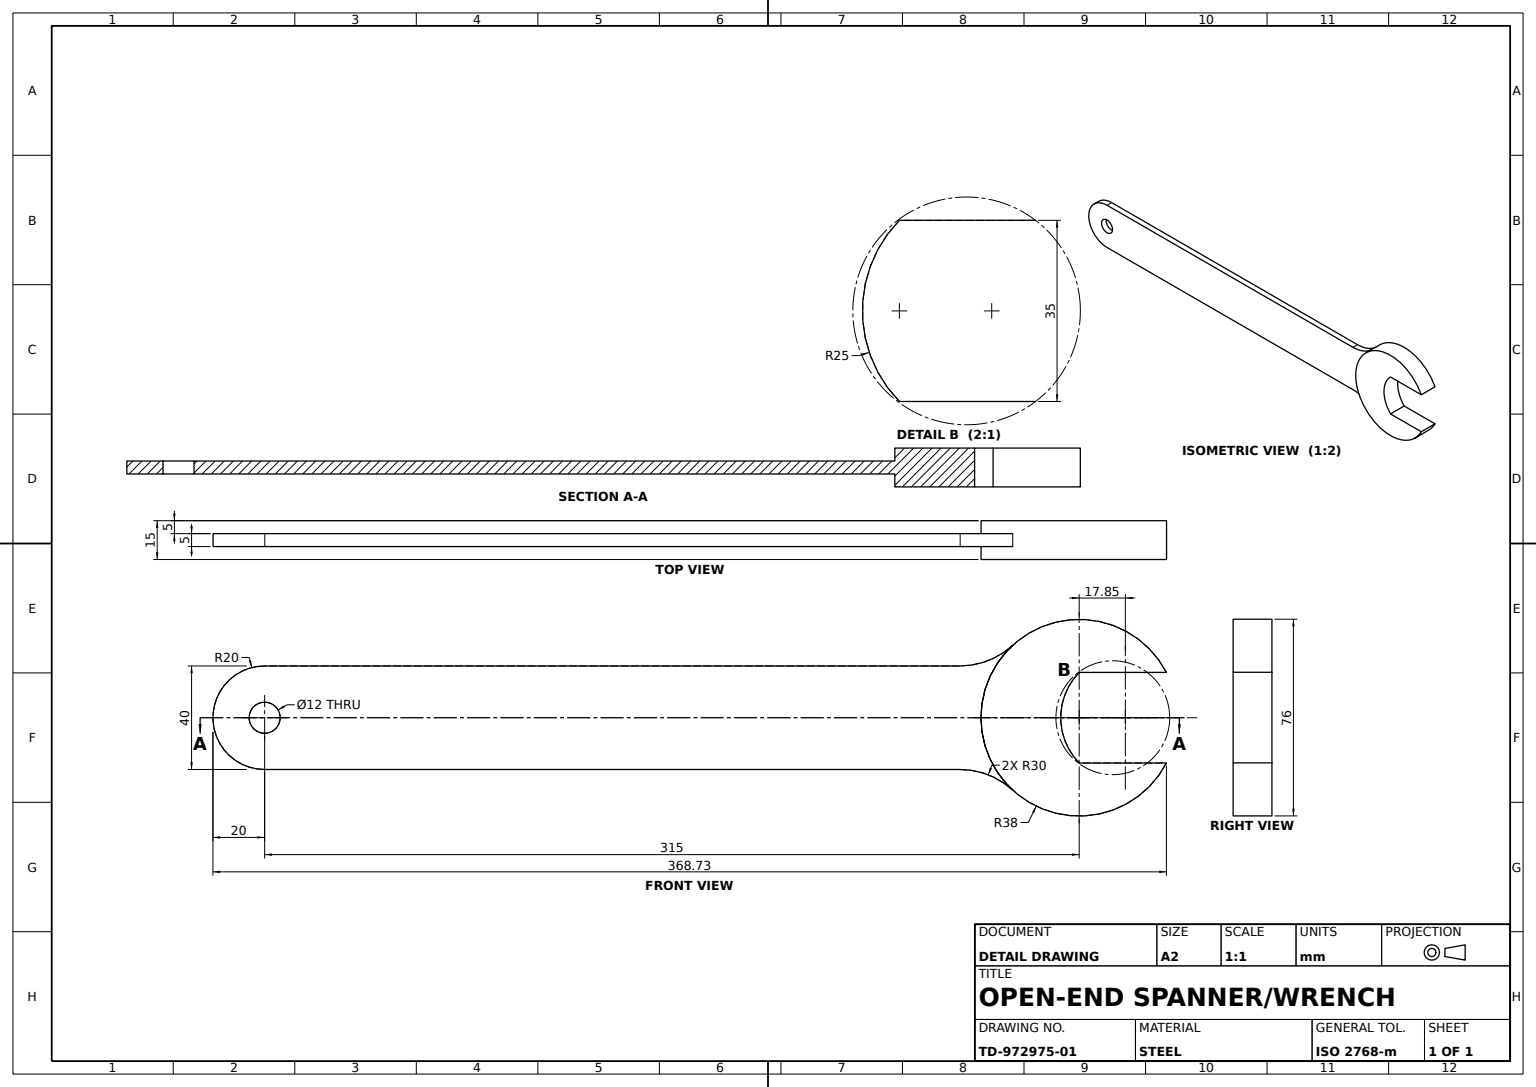
SolidWorks part; units mm, degrees
material "Plain Carbon Steel"
ref_plane "Front Plane" through (0, 0, 0) normal (0, 0, 1) x (1, 0, 0)
ref_plane "Top Plane" through (0, 0, 0) normal (0, 1, 0) x (1, 0, 0)
ref_plane "Right Plane" through (0, 0, 0) normal (1, 0, 0) x (0, 0, -1)
sketch "Handle Profile Sketch" plane through (0, 0, 0) normal (0, 0, 1) x (1, 0, 0)
  line L0 (0, 0) -> (315, 0)
  line L1 (315, 0) -> (315, 40)
  line L2 (315, 40) -> (0, 40)
  line L3 (0, 40) -> (0, 0)
  dimension "D2" = 40
  dimension "D1" = 315
  dimension "D3" = 315
extrude "Handle Bar 315x40x5" add sketch "Handle Profile Sketch" along normal blind 5
sketch "Hanging End Sketch" plane through (0, 0, 5) normal (0, 0, 1) x (1, 0, 0)
  line L0 (0, 40) -> (0, 0) construction
  circle A0 centre (0, 20) radius 20
  dimension "D1" = 20
extrude "Rounded Hanging End" add sketch "Hanging End Sketch" against normal blind 5
sketch "Neck Profile Sketch" plane through (0, 0, 5) normal (0, 0, 1) x (1, 0, 0)
  line L0 (315, 20) -> (281, 20)
  line L1 (315, 0) -> (315, 40) construction
  line L2 (315, 20) -> (315, 37.5)
  line L3 (315, 20) -> (315, 2.5)
  line L4 (315, 37.5) -> (348.7305, 37.5)
  line L5 (315, 2.5) -> (348.7305, 2.5)
  arc A0 (348.7305, 37.5) -> (348.7305, 2.5) centre (315, 20) ccw
  dimension "D4" = 38
  dimension "D1" = 34
  dimension "D2" = 17.5
  dimension "D3" = 17.5
extrude "Head Neck Boss" add sketch "Neck Profile Sketch" against normal blind 5
sketch "Neck Trim Sketch R25" plane through (0, 0, 5) normal (0, 0, 1) x (1, 0, 0)
  line L0 (315, 37.5) -> (315, 2.5)
  arc A0 (315, 37.5) -> (315, 2.5) centre (332.8536, 20) ccw
  dimension "D1" = 25
extrude "Neck Trim Cut R25" cut sketch "Neck Trim Sketch R25" against normal blind 5
sketch "Neck Fill Sketch A" plane through (0, 0, 5) normal (0, 0, 1) x (1, 0, 0)
  line L0 (348.7305, 37.5) -> (315, 37.5)
  line L1 (348.7305, 2.5) -> (315, 2.5)
  arc A0 (348.7305, 37.5) -> (348.7305, 2.5) centre (315, 20) ccw
  arc A1 (315, 37.5) -> (315, 2.5) centre (332.8536, 20) ccw
extrude "Neck Fill Boss A" add sketch "Neck Fill Sketch A" along normal blind 5
sketch "Neck Fill Sketch B" plane through (0, 0, 0) normal (0, 0, -1) x (-1, 0, 0)
  line L0 (-348.7305, 37.5) -> (-315, 37.5)
  line L1 (-348.7305, 2.5) -> (-315, 2.5)
  arc A0 (-348.7305, 2.5) -> (-348.7305, 37.5) centre (-315, 20) ccw
  arc A1 (-315, 2.5) -> (-315, 37.5) centre (-332.8536, 20) ccw
extrude "Neck Fill Boss B" add sketch "Neck Fill Sketch B" along normal blind 5
sketch "Jaw Head Sketch" plane through (0, 0, 0) normal (0, 0, -1) x (-1, 0, 0)
  line L0 (-282.689, 40) -> (0, 40) construction
  line L1 (0, 0) -> (-282.689, 0) construction
  line L2 (-268.9131, 40) -> (-282.689, 40)
  line L3 (-268.9131, 0) -> (-282.689, 0)
  arc A0 (-268.9131, 40) -> (-289.2456, 47.9412) centre (-268.9131, 70) cw
  arc A1 (-348.7305, 2.5) -> (-348.7305, 37.5) centre (-315, 20) ccw construction
  arc A2 (-289.2456, -7.9412) -> (-268.9131, 0) centre (-268.9131, -30) cw
  arc A3 (-289.2456, -7.9412) -> (-282.689, 0) centre (-315, 20) ccw
  arc A4 (-282.689, 40) -> (-289.2456, 47.9412) centre (-315, 20) ccw
  dimension "D1" = 30
  dimension "D2" = 30
extrude "Open Jaw Head" add sketch "Jaw Head Sketch" against normal blind 5
sketch "Hanging Hole Sketch" plane through (0, 0, 0) normal (0, 0, -1) x (-1, 0, 0)
  circle A1 centre (0, 20) radius 6
  dimension "D2" = 6
extrude "Hanging Hole Ø6" cut sketch "Hanging Hole Sketch" against normal blind 15
